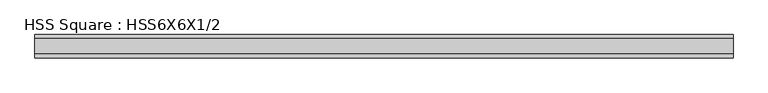
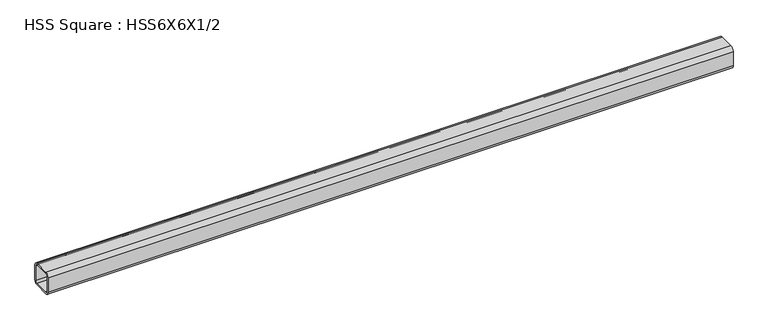
"""IFC4 building model written with IfcOpenShell, lengths in millimetres: member geometry, HSS Square : HSS6X6X1/2."""

from ifc_helpers import new_model, si_unit, point, frame, frame_2d, origin, place, context, project, spatial, polyline, circle_curve, trimmed, segment, composite_curve, outline, extrude, source, transform, mapped, element, save


def hss_square_hss6x6x1_2_f3b36863(model_context):
    return source(origin(), model_context, "Body", "SweptSolid", [
        extrude(outline(composite_curve([segment(trimmed(circle_curve(frame_2d((-50.8, 50.8)), 25.4), [point((-76.2, 50.8))], [point((-50.8, 76.2))], False, "CARTESIAN"), True, "CONTINUOUS"), segment(polyline([(-50.8, 76.2), (50.8, 76.2)]), True, "CONTINUOUS"), segment(trimmed(circle_curve(frame_2d((50.8, 50.8)), 25.4), [point((50.8, 76.2))], [point((76.2, 50.8))], False, "CARTESIAN"), True, "CONTINUOUS"), segment(polyline([(76.2, 50.8), (76.2, -50.8)]), True, "CONTINUOUS"), segment(trimmed(circle_curve(frame_2d((50.8, -50.8)), 25.4), [point((76.2, -50.8))], [point((50.8, -76.2))], False, "CARTESIAN"), True, "CONTINUOUS"), segment(polyline([(50.8, -76.2), (-50.8, -76.2)]), True, "CONTINUOUS"), segment(trimmed(circle_curve(frame_2d((-50.8, -50.8)), 25.4), [point((-50.8, -76.2))], [point((-76.2, -50.8))], False, "CARTESIAN"), True, "CONTINUOUS"), segment(polyline([(-76.2, -50.8), (-76.2, 50.8)]), True, "CONTINUOUS")], self_intersect=False), holes=[composite_curve([segment(polyline([(50.8, 63.5), (-50.8, 63.5)]), True, "CONTINUOUS"), segment(trimmed(circle_curve(frame_2d((-50.8, 50.8)), 12.7), [point((-50.8, 63.5))], [point((-63.5, 50.8))], True, "CARTESIAN"), True, "CONTINUOUS"), segment(polyline([(-63.5, 50.8), (-63.5, -50.8)]), True, "CONTINUOUS"), segment(trimmed(circle_curve(frame_2d((-50.8, -50.8)), 12.7), [point((-63.5, -50.8))], [point((-50.8, -63.5))], True, "CARTESIAN"), True, "CONTINUOUS"), segment(polyline([(-50.8, -63.5), (50.8, -63.5)]), True, "CONTINUOUS"), segment(trimmed(circle_curve(frame_2d((50.8, -50.8)), 12.7), [point((50.8, -63.5))], [point((63.5, -50.8))], True, "CARTESIAN"), True, "CONTINUOUS"), segment(polyline([(63.5, -50.8), (63.5, 50.8)]), True, "CONTINUOUS"), segment(trimmed(circle_curve(frame_2d((50.8, 50.8)), 12.7), [point((63.5, 50.8))], [point((50.8, 63.5))], True, "CARTESIAN"), True, "CONTINUOUS")], self_intersect=False)]), frame((-2402.8888982, 0.0, 0.0), z_axis=(1.0, 0.0, 0.0), x_axis=(0.0, 1.0, 0.0)), (0.0, 0.0, 1.0), 4587.7146296),
    ])


if __name__ == "__main__":
    model = new_model("IFC4")
    model_context = context("Model", 3, world=origin())
    ifc_project = project(units=[si_unit("LENGTHUNIT", "METRE", prefix="MILLI")], contexts=[model_context])
    site = spatial("IfcSite", under=ifc_project)
    building = spatial("IfcBuilding", under=site)
    placement = place(None, origin())
    hss_square_hss6x6x1_2_shape = hss_square_hss6x6x1_2_f3b36863(model_context)
    element("IfcMember", 1, ObjectType="HSS Square : HSS6X6X1/2", at=placement, inside=building, context=model_context, shape_type="MappedRepresentation", body=[
        mapped(hss_square_hss6x6x1_2_shape, transform((0.0, 0.0, 0.0), x_axis=(1.0, 0.0, 0.0), y_axis=(0.0, 1.0, 0.0), z_axis=(0.0, 0.0, 1.0))),
    ])
    save(model, "model.ifc")

# Revit data of these elements
# Type "HSS Square : HSS6X6X1/2"
#   Section Name Key = "HSS 6X6X1/2"
#   Assembly Code = "B10"
#   Width = 6.000"
#   Wall Nominal Thickness = 0.500"
#   Wall Design Thickness = 0.465"
#   Torsional Moment of Inertia = 81.10 in⁴
#   Torsional Modulus = 28.10 in³
#   Section Area = 9.74 in²
#   Plastic Modulus weak axis = 19.80 in³
#   Plastic Modulus strong axis = 19.80 in³
#   Outer Fillet = 1.000"
#   Nominal Weight = 35.24 lbf/ft
#   Moment of Inertia weak axis = 48.30 in⁴
#   Moment of Inertia strong axis = 48.30 in⁴
#   Inner Fillet = 0.500"
#   Height = 6.000"
#   Elastic Modulus weak axis = 16.10 in³
#   Elastic Modulus strong axis = 16.10 in³
#   Centroid Vertical = 3.000"
#   Centroid Horizontal = 3.000"
#   Length [instance default] = 5' - 0"
#   Structural Material [instance default] = Steel ASTM A500, Grade B, Rectangular and Square
#   Principal Axes Angle = 0
# Element 1 (IfcMember, "HSS Square : HSS6X6X1/2")
#   Structural Material = Steel ASTM A992
#   Materials on its faces: "Steel ASTM A992"
# Materials
#   "Steel ASTM A500, Grade B, Rectangular and Square": class "Metal", colour RGB 199 199 199, transparency 0, Description = "Carbon steel", Cost = 0
#   "Steel ASTM A992": class "Metal", colour RGB 199 199 199, transparency 0, Description = "Structural steel 50ksi", Cost = 0
